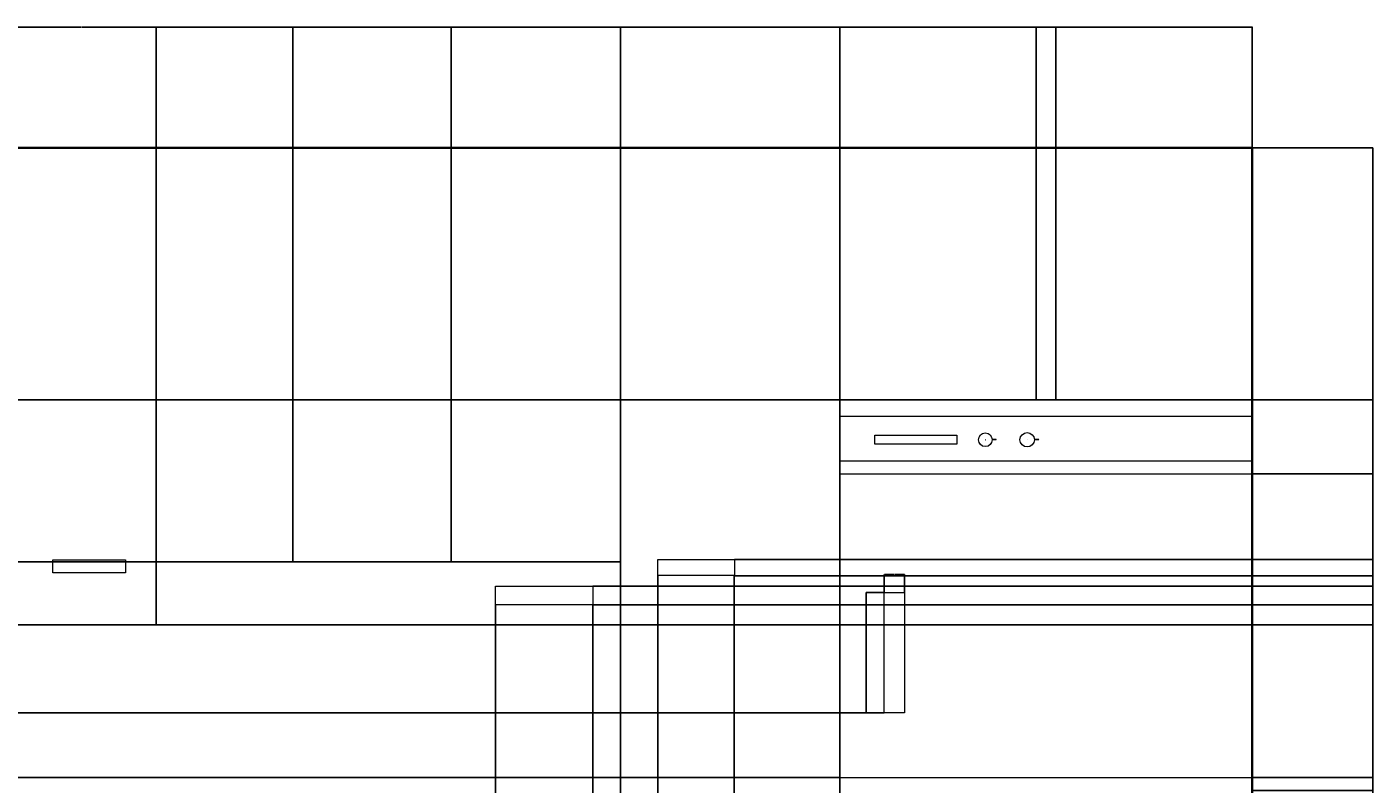
# Model space of a CAD drawing. Units: millimetres. Extents: x 4725 to 8727, y 2935 to 5260.
# Tile 3 of 3: x 6642 to 8727, y 4087 to 5260. Entities that reach past the tile are written whole.
import ezdxf

# ---------------------------------------------------------------- set-up
doc = ezdxf.new("R2010")
doc.units = ezdxf.units.MM
for name, color, linetype, lineweight in [('A-ANNO-DIMS', 2, 'Continuous', 18), ('A-CASE-HRDW', 9, 'Continuous', 13), ('A-ELEV', 7, 'Continuous', 35), ('A-EQPM', 4, 'Continuous', 18), ('A-FLOR-CASE', 8, 'Continuous', 25)]:
    doc.layers.add(name, color=color, linetype=linetype, lineweight=lineweight)
doc.styles.get("Standard").update_dxf_attribs({"font": 'arial.ttf'})
doc.dimstyles.get("Standard").update_dxf_attribs({"dimtxt": 0.18, "dimasz": 0.18, "dimexe": 0.18, "dimexo": 0.0625, "dimgap": 0.09, "dimtad": 0, "dimtih": 1, "dimtoh": 1, "dimdec": 4, "dimzin": 0, "dimdsep": 46, "dimtxsty": 'Standard', "dimcen": 0.09, "dimadec": 0, "dimazin": 0, "dimtfac": 1, "dimtdec": 4, "dimtofl": 0, "dimtmove": 0, "dimatfit": 3, "dimfxl": 1, "dimtolj": 1, "dimtzin": 0, "dimarcsym": 0})

# ---------------------------------------------------------------- blocks, each defined once
blk = doc.blocks.new('REFRIGERATOR-DOOR-PULL')
blk.add_lwpolyline([(0, 186.1), (31.3, 186.1), (31.3, 0), (0, 0)], close=True)
blk = doc.blocks.new('*D5')
at = {"layer": 'A-ANNO-DIMS', "color": 0, "lineweight": -2, "transparency": 16777216}
for p, q in [((7969.7, 4384.1), (7941.7, 4384.1)), ((7941.9, 4383.9), (7941.9, 4291.2)), ((7941.9, 4198.2), (7941.9, 4290.9)), ((7969.7, 4198), (7941.7, 4198))]:
    blk.add_line(p, q, dxfattribs=at)
at = {"layer": 'A-ANNO-DIMS', "color": 0, "transparency": 16777216}
for points in [[(7941.8, 4383.9), (7941.9, 4383.9), (7941.9, 4384.1)], [(7941.8, 4198.2), (7941.9, 4198.2), (7941.9, 4198)]]:
    blk.add_solid(points, dxfattribs=at)
at = {"layer": 'Defpoints', "color": 0, "transparency": 16777216}
for p in [(7941.9, 4384.1), (7969.8, 4384.1), (7969.8, 4198)]:
    blk.add_point(p, dxfattribs=at)
at = {"layer": 'A-ANNO-DIMS', "color": 0, "transparency": 16777216, "insert": (7941.9, 4291), "char_height": 0.18, "attachment_point": 5}
blk.add_mtext('\\A1;PULL 186 TYP.', dxfattribs=at)
blk = doc.blocks.new('*D6')
at = {"layer": 'A-ANNO-DIMS', "color": 0, "lineweight": -2, "transparency": 16777216}
for p, q in [((7969.8, 4384.1), (7969.8, 4412.2)), ((7969.9, 4412), (7984.9, 4412)), ((8000.9, 4412), (7985.9, 4412)), ((8001, 4384.1), (8001, 4412.2))]:
    blk.add_line(p, q, dxfattribs=at)
at = {"layer": 'A-ANNO-DIMS', "color": 0, "transparency": 16777216}
for points in [[(7969.9, 4412), (7969.9, 4412), (7969.8, 4412)], [(8000.9, 4412), (8000.9, 4412), (8001, 4412)]]:
    blk.add_solid(points, dxfattribs=at)
at = {"layer": 'Defpoints', "color": 0, "transparency": 16777216}
for p in [(8001, 4412), (7969.8, 4384.1), (8001, 4384.1)]:
    blk.add_point(p, dxfattribs=at)
at = {"layer": 'A-ANNO-DIMS', "color": 0, "transparency": 16777216, "insert": (7985.4, 4412), "char_height": 0.18, "attachment_point": 5}
blk.add_mtext('\\A1;31 TYP.', dxfattribs=at)
blk = doc.blocks.new('*D14')
at = {"layer": 'A-ANNO-DIMS', "color": 0, "lineweight": -2, "transparency": 16777216}
for p, q in [((6841.9, 5073.2), (6841.9, 5260.1)), ((6842.1, 5260), (6947.4, 5260)), ((7053.5, 5260), (6948.2, 5260)), ((7053.7, 5073.2), (7053.7, 5260.1))]:
    blk.add_line(p, q, dxfattribs=at)
at = {"layer": 'A-ANNO-DIMS', "color": 0, "transparency": 16777216}
for points in [[(6842.1, 5260), (6842.1, 5259.9), (6841.9, 5260)], [(7053.5, 5260), (7053.5, 5259.9), (7053.7, 5260)]]:
    blk.add_solid(points, dxfattribs=at)
at = {"layer": 'Defpoints', "color": 0, "transparency": 16777216}
for p in [(7053.7, 5260), (6841.9, 5073.1), (7053.7, 5073.1)]:
    blk.add_point(p, dxfattribs=at)
at = {"layer": 'A-ANNO-DIMS', "color": 0, "transparency": 16777216, "insert": (6947.8, 5260), "char_height": 0.18, "attachment_point": 5}
blk.add_mtext('\\A1;211.8', dxfattribs=at)
blk = doc.blocks.new('*D15')
at = {"layer": 'A-ANNO-DIMS', "color": 0, "lineweight": -2, "transparency": 16777216}
for p, q in [((7053.7, 5073.2), (7053.7, 5260.1)), ((7053.9, 5260), (7176, 5260)), ((7298.9, 5260), (7176.8, 5260)), ((7299.1, 5073.2), (7299.1, 5260.1))]:
    blk.add_line(p, q, dxfattribs=at)
at = {"layer": 'A-ANNO-DIMS', "color": 0, "transparency": 16777216}
for points in [[(7053.9, 5260), (7053.9, 5259.9), (7053.7, 5260)], [(7298.9, 5260), (7298.9, 5259.9), (7299.1, 5260)]]:
    blk.add_solid(points, dxfattribs=at)
at = {"layer": 'Defpoints', "color": 0, "transparency": 16777216}
for p in [(7299.1, 5260), (7053.7, 5073.1), (7299.1, 5073.1)]:
    blk.add_point(p, dxfattribs=at)
at = {"layer": 'A-ANNO-DIMS', "color": 0, "transparency": 16777216, "insert": (7176.4, 5260), "char_height": 0.18, "attachment_point": 5}
blk.add_mtext('\\A1;245.4', dxfattribs=at)
blk = doc.blocks.new('*D16')
at = {"layer": 'A-ANNO-DIMS', "color": 0, "lineweight": -2, "transparency": 16777216}
for p, q in [((7299.1, 5073.2), (7299.1, 5260.1)), ((7299.3, 5260), (7429.8, 5260)), ((7561.2, 5260), (7430.6, 5260)), ((7561.3, 5073.2), (7561.3, 5260.1))]:
    blk.add_line(p, q, dxfattribs=at)
at = {"layer": 'A-ANNO-DIMS', "color": 0, "transparency": 16777216}
for points in [[(7299.3, 5260), (7299.3, 5259.9), (7299.1, 5260)], [(7561.2, 5260), (7561.2, 5259.9), (7561.3, 5260)]]:
    blk.add_solid(points, dxfattribs=at)
at = {"layer": 'Defpoints', "color": 0, "transparency": 16777216}
for p in [(7561.3, 5260), (7299.1, 5073.1), (7561.3, 5073.1)]:
    blk.add_point(p, dxfattribs=at)
at = {"layer": 'A-ANNO-DIMS', "color": 0, "transparency": 16777216, "insert": (7430.2, 5260), "char_height": 0.18, "attachment_point": 5}
blk.add_mtext('\\A1;262.2', dxfattribs=at)
blk = doc.blocks.new('*D17')
at = {"layer": 'A-ANNO-DIMS', "color": 0, "lineweight": -2, "transparency": 16777216}
for p, q in [((7561.3, 5073.2), (7561.3, 5260.1)), ((7561.5, 5260), (7730.7, 5260)), ((7900.7, 5260), (7731.5, 5260)), ((7900.9, 5073.2), (7900.9, 5260.1))]:
    blk.add_line(p, q, dxfattribs=at)
at = {"layer": 'A-ANNO-DIMS', "color": 0, "transparency": 16777216}
for points in [[(7561.5, 5260), (7561.5, 5259.9), (7561.3, 5260)], [(7900.7, 5260), (7900.7, 5259.9), (7900.9, 5260)]]:
    blk.add_solid(points, dxfattribs=at)
at = {"layer": 'Defpoints', "color": 0, "transparency": 16777216}
for p in [(7900.9, 5260), (7561.3, 5073.1), (7900.9, 5073.1)]:
    blk.add_point(p, dxfattribs=at)
at = {"layer": 'A-ANNO-DIMS', "color": 0, "transparency": 16777216, "insert": (7731.1, 5260), "char_height": 0.18, "attachment_point": 5}
blk.add_mtext('\\A1;339.5', dxfattribs=at)
blk = doc.blocks.new('*D18')
at = {"layer": 'A-ANNO-DIMS', "color": 0, "lineweight": -2, "transparency": 16777216}
for p, q in [((7900.9, 5073.2), (7900.9, 5260.1)), ((7901, 5260), (8052.6, 5260)), ((8205, 5260), (8053.5, 5260)), ((8205.2, 5073.2), (8205.2, 5260.1))]:
    blk.add_line(p, q, dxfattribs=at)
at = {"layer": 'A-ANNO-DIMS', "color": 0, "transparency": 16777216}
for points in [[(7901, 5260), (7901, 5259.9), (7900.9, 5260)], [(8205, 5260), (8205, 5259.9), (8205.2, 5260)]]:
    blk.add_solid(points, dxfattribs=at)
at = {"layer": 'Defpoints', "color": 0, "transparency": 16777216}
for p in [(8205.2, 5260), (7900.9, 5073.1), (8205.2, 5073.1)]:
    blk.add_point(p, dxfattribs=at)
at = {"layer": 'A-ANNO-DIMS', "color": 0, "transparency": 16777216, "insert": (8053, 5260), "char_height": 0.18, "attachment_point": 5}
blk.add_mtext('\\A1;304.35', dxfattribs=at)
blk = doc.blocks.new('*D19')
at = {"layer": 'A-ANNO-DIMS', "color": 0, "lineweight": -2, "transparency": 16777216}
for p, q in [((8205.2, 5073.2), (8205.2, 5260.1)), ((8205.4, 5260), (8220, 5260)), ((8235, 5260), (8220.4, 5260)), ((8235.2, 5073.2), (8235.2, 5260.1))]:
    blk.add_line(p, q, dxfattribs=at)
at = {"layer": 'A-ANNO-DIMS', "color": 0, "transparency": 16777216}
for points in [[(8205.4, 5260), (8205.4, 5259.9), (8205.2, 5260)], [(8235, 5260), (8235, 5259.9), (8235.2, 5260)]]:
    blk.add_solid(points, dxfattribs=at)
at = {"layer": 'Defpoints', "color": 0, "transparency": 16777216}
for p in [(8235.2, 5260), (8205.2, 5073.1), (8235.2, 5073.1)]:
    blk.add_point(p, dxfattribs=at)
at = {"layer": 'A-ANNO-DIMS', "color": 0, "transparency": 16777216, "insert": (8220.2, 5260), "char_height": 0.18, "attachment_point": 5}
blk.add_mtext('\\A1;30', dxfattribs=at)
blk = doc.blocks.new('*D20')
at = {"layer": 'A-ANNO-DIMS', "color": 0, "lineweight": -2, "transparency": 16777216}
for p, q in [((8235.2, 5073.2), (8235.2, 5260.1)), ((8235.4, 5260), (8386.9, 5260)), ((8539.4, 5260), (8387.9, 5260)), ((8539.6, 5073.2), (8539.6, 5260.1))]:
    blk.add_line(p, q, dxfattribs=at)
at = {"layer": 'A-ANNO-DIMS', "color": 0, "transparency": 16777216}
for points in [[(8235.4, 5260), (8235.4, 5259.9), (8235.2, 5260)], [(8539.4, 5260), (8539.4, 5259.9), (8539.6, 5260)]]:
    blk.add_solid(points, dxfattribs=at)
at = {"layer": 'Defpoints', "color": 0, "transparency": 16777216}
for p in [(8539.6, 5260), (8235.2, 5073.1), (8539.6, 5073.1)]:
    blk.add_point(p, dxfattribs=at)
at = {"layer": 'A-ANNO-DIMS', "color": 0, "transparency": 16777216, "insert": (8387.4, 5260), "char_height": 0.18, "attachment_point": 5}
blk.add_mtext('\\A1;304.35', dxfattribs=at)
blk = doc.blocks.new('*D27')
at = {"layer": 'A-ANNO-DIMS', "color": 0, "lineweight": -2, "transparency": 16777216}
for p, q in [((8539.6, 4097.4), (8726.6, 4097.4)), ((8726.4, 4097.2), (8726.4, 4087.6)), ((8726.4, 4077.6), (8726.4, 4087.2)), ((8539.6, 4077.4), (8726.6, 4077.4))]:
    blk.add_line(p, q, dxfattribs=at)
at = {"layer": 'A-ANNO-DIMS', "color": 0, "transparency": 16777216}
for points in [[(8726.4, 4097.2), (8726.4, 4097.2), (8726.4, 4097.4)], [(8726.4, 4077.6), (8726.4, 4077.6), (8726.4, 4077.4)]]:
    blk.add_solid(points, dxfattribs=at)
at = {"layer": 'Defpoints', "color": 0, "transparency": 16777216}
for p in [(8539.6, 4097.4), (8726.4, 4097.4), (8539.6, 4077.4)]:
    blk.add_point(p, dxfattribs=at)
at = {"layer": 'A-ANNO-DIMS', "color": 0, "transparency": 16777216, "insert": (8726.4, 4087.4), "char_height": 0.18, "attachment_point": 5}
blk.add_mtext('\\A1;20', dxfattribs=at)
blk = doc.blocks.new('*D28')
at = {"layer": 'A-ANNO-DIMS', "color": 0, "lineweight": -2, "transparency": 16777216}
for p, q in [((8539.6, 4568), (8726.6, 4568)), ((8726.4, 4567.8), (8726.4, 4332.9)), ((8726.4, 4097.6), (8726.4, 4332.5)), ((8539.6, 4097.4), (8726.6, 4097.4))]:
    blk.add_line(p, q, dxfattribs=at)
at = {"layer": 'A-ANNO-DIMS', "color": 0, "transparency": 16777216}
for points in [[(8726.4, 4567.8), (8726.4, 4567.8), (8726.4, 4568)], [(8726.4, 4097.6), (8726.4, 4097.6), (8726.4, 4097.4)]]:
    blk.add_solid(points, dxfattribs=at)
at = {"layer": 'Defpoints', "color": 0, "transparency": 16777216}
for p in [(8539.6, 4568), (8539.6, 4097.4), (8726.4, 4097.4)]:
    blk.add_point(p, dxfattribs=at)
at = {"layer": 'A-ANNO-DIMS', "color": 0, "transparency": 16777216, "insert": (8726.4, 4332.7), "char_height": 0.18, "attachment_point": 5}
blk.add_mtext('\\A1;470.6', dxfattribs=at)
blk = doc.blocks.new('*D29')
at = {"layer": 'A-ANNO-DIMS', "color": 0, "lineweight": -2, "transparency": 16777216}
for p, q in [((8539.6, 4682.5), (8726.6, 4682.5)), ((8726.4, 4682.3), (8726.4, 4625.4)), ((8726.4, 4568.2), (8726.4, 4625)), ((8539.6, 4568), (8726.6, 4568))]:
    blk.add_line(p, q, dxfattribs=at)
at = {"layer": 'A-ANNO-DIMS', "color": 0, "transparency": 16777216}
for points in [[(8726.4, 4682.3), (8726.4, 4682.3), (8726.4, 4682.5)], [(8726.4, 4568.2), (8726.4, 4568.2), (8726.4, 4568)]]:
    blk.add_solid(points, dxfattribs=at)
at = {"layer": 'Defpoints', "color": 0, "transparency": 16777216}
for p in [(8539.6, 4682.5), (8726.4, 4682.5), (8539.6, 4568)]:
    blk.add_point(p, dxfattribs=at)
at = {"layer": 'A-ANNO-DIMS', "color": 0, "transparency": 16777216, "insert": (8726.4, 4625.2), "char_height": 0.18, "attachment_point": 5}
blk.add_mtext('\\A1;114.46', dxfattribs=at)
blk = doc.blocks.new('*D30')
at = {"layer": 'A-ANNO-DIMS', "color": 0, "lineweight": -2, "transparency": 16777216}
for p, q in [((8205.1, 5073.1), (4725.3, 5073.1)), ((4725.5, 5072.9), (4725.5, 4878)), ((4725.5, 4682.6), (4725.5, 4877.6)), ((7900.8, 4682.5), (4725.3, 4682.5))]:
    blk.add_line(p, q, dxfattribs=at)
at = {"layer": 'A-ANNO-DIMS', "color": 0, "transparency": 16777216}
for points in [[(4725.5, 5072.9), (4725.5, 5072.9), (4725.5, 5073.1)], [(4725.5, 4682.6), (4725.5, 4682.6), (4725.5, 4682.5)]]:
    blk.add_solid(points, dxfattribs=at)
at = {"layer": 'Defpoints', "color": 0, "transparency": 16777216}
for p in [(4725.5, 5073.1), (8205.2, 5073.1), (7900.9, 4682.5)]:
    blk.add_point(p, dxfattribs=at)
at = {"layer": 'A-ANNO-DIMS', "color": 0, "transparency": 16777216, "insert": (4725.5, 4877.8), "char_height": 0.18, "attachment_point": 5}
blk.add_mtext('\\A1;390.7', dxfattribs=at)
blk = doc.blocks.new('*D31')
at = {"layer": 'A-ANNO-DIMS', "color": 0, "lineweight": -2, "transparency": 16777216}
for p, q in [((6841.9, 4431.6), (4725.3, 4431.6)), ((4725.5, 4431.4), (4725.5, 4383.1)), ((4725.5, 4334.4), (4725.5, 4382.7)), ((6841.9, 4334.2), (4725.3, 4334.2))]:
    blk.add_line(p, q, dxfattribs=at)
at = {"layer": 'A-ANNO-DIMS', "color": 0, "transparency": 16777216}
for points in [[(4725.5, 4431.4), (4725.5, 4431.4), (4725.5, 4431.6)], [(4725.5, 4334.4), (4725.5, 4334.4), (4725.5, 4334.2)]]:
    blk.add_solid(points, dxfattribs=at)
at = {"layer": 'Defpoints', "color": 0, "transparency": 16777216}
for p in [(4725.5, 4431.6), (6841.9, 4431.6), (6841.9, 4334.2)]:
    blk.add_point(p, dxfattribs=at)
at = {"layer": 'A-ANNO-DIMS', "color": 0, "transparency": 16777216, "insert": (4725.5, 4382.9), "char_height": 0.18, "attachment_point": 5}
blk.add_mtext('\\A1;97.4', dxfattribs=at)
blk = doc.blocks.new('*D32')
at = {"layer": 'A-ANNO-DIMS', "color": 0, "lineweight": -2, "transparency": 16777216}
for p, q in [((7367.7, 4364.8), (7367.7, 2934.7)), ((7518.4, 4364.8), (7518.4, 2934.7)), ((7367.8, 2934.8), (7442.6, 2934.8)), ((7518.2, 2934.8), (7443.5, 2934.8))]:
    blk.add_line(p, q, dxfattribs=at)
at = {"layer": 'A-ANNO-DIMS', "color": 0, "transparency": 16777216}
for points in [[(7367.8, 2934.9), (7367.8, 2934.8), (7367.7, 2934.8)], [(7518.2, 2934.9), (7518.2, 2934.8), (7518.4, 2934.8)]]:
    blk.add_solid(points, dxfattribs=at)
at = {"layer": 'Defpoints', "color": 0, "transparency": 16777216}
for p in [(7367.7, 4364.8), (7518.4, 4364.8), (7518.4, 2934.8)]:
    blk.add_point(p, dxfattribs=at)
at = {"layer": 'A-ANNO-DIMS', "color": 0, "transparency": 16777216, "insert": (7443, 2934.8), "char_height": 0.18, "attachment_point": 5}
blk.add_mtext('\\A1;150.77', dxfattribs=at)
blk = doc.blocks.new('*D33')
at = {"layer": 'A-ANNO-DIMS', "color": 0, "lineweight": -2, "transparency": 16777216}
for p, q in [((7518.4, 4364.8), (7518.4, 2934.7)), ((7561.3, 4334.1), (7561.3, 2934.7)), ((7518.6, 2934.8), (7539.4, 2934.8)), ((7561.2, 2934.8), (7540.3, 2934.8))]:
    blk.add_line(p, q, dxfattribs=at)
at = {"layer": 'A-ANNO-DIMS', "color": 0, "transparency": 16777216}
for points in [[(7518.6, 2934.9), (7518.6, 2934.8), (7518.4, 2934.8)], [(7561.2, 2934.9), (7561.2, 2934.8), (7561.3, 2934.8)]]:
    blk.add_solid(points, dxfattribs=at)
at = {"layer": 'Defpoints', "color": 0, "transparency": 16777216}
for p in [(7518.4, 4364.8), (7561.3, 4334.2), (7561.3, 2934.8)]:
    blk.add_point(p, dxfattribs=at)
at = {"layer": 'A-ANNO-DIMS', "color": 0, "transparency": 16777216, "insert": (7539.9, 2934.8), "char_height": 0.18, "attachment_point": 5}
blk.add_mtext('\\A1;42.905', dxfattribs=at)
blk = doc.blocks.new('*D34')
at = {"layer": 'A-ANNO-DIMS', "color": 0, "lineweight": -2, "transparency": 16777216}
for p, q in [((7619, 4410.2), (7619, 2934.7)), ((7737.5, 4410.2), (7737.5, 2934.7)), ((7619.2, 2934.8), (7677.8, 2934.8)), ((7737.4, 2934.8), (7678.7, 2934.8))]:
    blk.add_line(p, q, dxfattribs=at)
at = {"layer": 'A-ANNO-DIMS', "color": 0, "transparency": 16777216}
for points in [[(7619.2, 2934.9), (7619.2, 2934.8), (7619, 2934.8)], [(7737.4, 2934.9), (7737.4, 2934.8), (7737.5, 2934.8)]]:
    blk.add_solid(points, dxfattribs=at)
at = {"layer": 'Defpoints', "color": 0, "transparency": 16777216}
for p in [(7619, 4410.2), (7737.5, 4410.2), (7737.5, 2934.8)]:
    blk.add_point(p, dxfattribs=at)
at = {"layer": 'A-ANNO-DIMS', "color": 0, "transparency": 16777216, "insert": (7678.3, 2934.8), "char_height": 0.18, "attachment_point": 5}
blk.add_mtext('\\A1;118.53', dxfattribs=at)
blk = doc.blocks.new('*D35')
at = {"layer": 'A-ANNO-DIMS', "color": 0, "lineweight": -2, "transparency": 16777216}
for p, q in [((7737.5, 4410.2), (7737.5, 2934.7)), ((7900.9, 4334.1), (7900.9, 2934.7)), ((7737.7, 2934.8), (7818.7, 2934.8)), ((7900.7, 2934.8), (7819.7, 2934.8))]:
    blk.add_line(p, q, dxfattribs=at)
at = {"layer": 'A-ANNO-DIMS', "color": 0, "transparency": 16777216}
for points in [[(7737.7, 2934.9), (7737.7, 2934.8), (7737.5, 2934.8)], [(7900.7, 2934.9), (7900.7, 2934.8), (7900.9, 2934.8)]]:
    blk.add_solid(points, dxfattribs=at)
at = {"layer": 'Defpoints', "color": 0, "transparency": 16777216}
for p in [(7737.5, 4410.2), (7900.9, 4334.2), (7900.9, 2934.8)]:
    blk.add_point(p, dxfattribs=at)
at = {"layer": 'A-ANNO-DIMS', "color": 0, "transparency": 16777216, "insert": (7819.2, 2934.8), "char_height": 0.18, "attachment_point": 5}
blk.add_mtext('\\A1;163.32', dxfattribs=at)
blk = doc.blocks.new('*D36')
at = {"layer": 'A-ANNO-DIMS', "color": 0, "lineweight": -2, "transparency": 16777216}
for p, q in [((7737.6, 4435.1), (8726.6, 4435.1)), ((8726.4, 4434.9), (8726.4, 4422.8)), ((8726.4, 4410.4), (8726.4, 4422.5)), ((7737.6, 4410.2), (8726.6, 4410.2))]:
    blk.add_line(p, q, dxfattribs=at)
at = {"layer": 'A-ANNO-DIMS', "color": 0, "transparency": 16777216}
for points in [[(8726.4, 4434.9), (8726.4, 4434.9), (8726.4, 4435.1)], [(8726.4, 4410.4), (8726.4, 4410.4), (8726.4, 4410.2)]]:
    blk.add_solid(points, dxfattribs=at)
at = {"layer": 'Defpoints', "color": 0, "transparency": 16777216}
for p in [(7737.5, 4435.1), (8726.4, 4435.1), (7737.5, 4410.2)]:
    blk.add_point(p, dxfattribs=at)
at = {"layer": 'A-ANNO-DIMS', "color": 0, "transparency": 16777216, "insert": (8726.4, 4422.7), "char_height": 0.18, "attachment_point": 5}
blk.add_mtext('\\A1;24.846', dxfattribs=at)
blk = doc.blocks.new('*D37')
at = {"layer": 'A-ANNO-DIMS', "color": 0, "lineweight": -2, "transparency": 16777216}
for p, q in [((7737.6, 4410.2), (8726.6, 4410.2)), ((8726.4, 4410.1), (8726.4, 4372.4)), ((8726.4, 4334.4), (8726.4, 4372)), ((7900.9, 4334.2), (8726.6, 4334.2))]:
    blk.add_line(p, q, dxfattribs=at)
at = {"layer": 'A-ANNO-DIMS', "color": 0, "transparency": 16777216}
for points in [[(8726.4, 4410.1), (8726.4, 4410.1), (8726.4, 4410.2)], [(8726.4, 4334.4), (8726.4, 4334.4), (8726.4, 4334.2)]]:
    blk.add_solid(points, dxfattribs=at)
at = {"layer": 'Defpoints', "color": 0, "transparency": 16777216}
for p in [(7737.5, 4410.2), (8726.4, 4410.2), (7900.9, 4334.2)]:
    blk.add_point(p, dxfattribs=at)
at = {"layer": 'A-ANNO-DIMS', "color": 0, "transparency": 16777216, "insert": (8726.4, 4372.2), "char_height": 0.18, "attachment_point": 5}
blk.add_mtext('\\A1;76.04', dxfattribs=at)
blk = doc.blocks.new('*D38')
at = {"layer": 'A-ANNO-DIMS', "color": 0, "lineweight": -2, "transparency": 16777216}
for p, q in [((7518.5, 4394.2), (8726.6, 4394.2)), ((8726.4, 4394), (8726.4, 4379.7)), ((8726.4, 4365), (8726.4, 4379.3)), ((7518.5, 4364.8), (8726.6, 4364.8))]:
    blk.add_line(p, q, dxfattribs=at)
at = {"layer": 'A-ANNO-DIMS', "color": 0, "transparency": 16777216}
for points in [[(8726.4, 4394), (8726.4, 4394), (8726.4, 4394.2)], [(8726.4, 4365), (8726.4, 4365), (8726.4, 4364.8)]]:
    blk.add_solid(points, dxfattribs=at)
at = {"layer": 'Defpoints', "color": 0, "transparency": 16777216}
for p in [(7518.4, 4394.2), (8726.4, 4394.2), (7518.4, 4364.8)]:
    blk.add_point(p, dxfattribs=at)
at = {"layer": 'A-ANNO-DIMS', "color": 0, "transparency": 16777216, "insert": (8726.4, 4379.5), "char_height": 0.18, "attachment_point": 5}
blk.add_mtext('\\A1;29.33', dxfattribs=at)
blk = doc.blocks.new('*D39')
at = {"layer": 'A-ANNO-DIMS', "color": 0, "lineweight": -2, "transparency": 16777216}
for p, q in [((7518.5, 4364.8), (8726.6, 4364.8)), ((8726.4, 4364.6), (8726.4, 4349.7)), ((8726.4, 4334.4), (8726.4, 4349.3)), ((7561.4, 4334.2), (8726.6, 4334.2))]:
    blk.add_line(p, q, dxfattribs=at)
at = {"layer": 'A-ANNO-DIMS', "color": 0, "transparency": 16777216}
for points in [[(8726.4, 4364.6), (8726.4, 4364.6), (8726.4, 4364.8)], [(8726.4, 4334.4), (8726.4, 4334.4), (8726.4, 4334.2)]]:
    blk.add_solid(points, dxfattribs=at)
at = {"layer": 'Defpoints', "color": 0, "transparency": 16777216}
for p in [(7518.4, 4364.8), (8726.4, 4364.8), (7561.3, 4334.2)]:
    blk.add_point(p, dxfattribs=at)
at = {"layer": 'A-ANNO-DIMS', "color": 0, "transparency": 16777216, "insert": (8726.4, 4349.5), "char_height": 0.18, "attachment_point": 5}
blk.add_mtext('\\A1;30.63', dxfattribs=at)
blk = doc.blocks.new('*D40')
at = {"layer": 'A-ANNO-DIMS', "color": 0, "lineweight": -2, "transparency": 16777216}
for p, q in [((4912.4, 5073.2), (4912.4, 5260.1)), ((4912.5, 5260), (6725.6, 5260)), ((8539.4, 5260), (6726.3, 5260)), ((8539.6, 5073.2), (8539.6, 5260.1))]:
    blk.add_line(p, q, dxfattribs=at)
at = {"layer": 'A-ANNO-DIMS', "color": 0, "transparency": 16777216}
for points in [[(4912.5, 5260), (4912.5, 5259.9), (4912.4, 5260)], [(8539.4, 5260), (8539.4, 5259.9), (8539.6, 5260)]]:
    blk.add_solid(points, dxfattribs=at)
at = {"layer": 'Defpoints', "color": 0, "transparency": 16777216}
for p in [(8539.6, 5260), (4912.4, 5073.1), (8539.6, 5073.1)]:
    blk.add_point(p, dxfattribs=at)
at = {"layer": 'A-ANNO-DIMS', "color": 0, "transparency": 16777216, "insert": (6726, 5260), "char_height": 0.18, "attachment_point": 5}
blk.add_mtext('\\A1;3627', dxfattribs=at)
blk = doc.blocks.new('*D41')
at = {"layer": 'A-ANNO-DIMS', "color": 0, "lineweight": -2, "transparency": 16777216}
for p, q in [((4912.4, 5073.1), (8726.6, 5073.1)), ((8726.4, 5072.9), (8726.4, 4097.6)), ((8726.4, 3121.9), (8726.4, 4097.2)), ((8539.6, 3121.7), (8726.6, 3121.7))]:
    blk.add_line(p, q, dxfattribs=at)
at = {"layer": 'A-ANNO-DIMS', "color": 0, "transparency": 16777216}
for points in [[(8726.4, 5072.9), (8726.4, 5072.9), (8726.4, 5073.1)], [(8726.4, 3121.9), (8726.4, 3121.9), (8726.4, 3121.7)]]:
    blk.add_solid(points, dxfattribs=at)
at = {"layer": 'Defpoints', "color": 0, "transparency": 16777216}
for p in [(4912.4, 5073.1), (8726.4, 5073.1), (8539.6, 3121.7)]:
    blk.add_point(p, dxfattribs=at)
at = {"layer": 'A-ANNO-DIMS', "color": 0, "transparency": 16777216, "insert": (8726.4, 4097.4), "char_height": 0.18, "attachment_point": 5}
blk.add_mtext('\\A1;1951.4', dxfattribs=at)
blk = doc.blocks.new('*D43')
at = {"layer": 'A-ANNO-DIMS', "color": 0, "lineweight": -2, "transparency": 16777216}
for p, q in [((7969.7, 4198), (4725.3, 4198)), ((4725.5, 4197.8), (4725.5, 4147.9)), ((4725.5, 4097.6), (4725.5, 4147.5)), ((7900.8, 4097.4), (4725.3, 4097.4))]:
    blk.add_line(p, q, dxfattribs=at)
at = {"layer": 'A-ANNO-DIMS', "color": 0, "transparency": 16777216}
for points in [[(4725.5, 4197.8), (4725.5, 4197.8), (4725.5, 4198)], [(4725.5, 4097.6), (4725.5, 4097.6), (4725.5, 4097.4)]]:
    blk.add_solid(points, dxfattribs=at)
at = {"layer": 'Defpoints', "color": 0, "transparency": 16777216}
for p in [(4725.5, 4198), (7969.8, 4198), (7900.9, 4097.4)]:
    blk.add_point(p, dxfattribs=at)
at = {"layer": 'A-ANNO-DIMS', "color": 0, "transparency": 16777216, "insert": (4725.5, 4147.7), "char_height": 0.18, "attachment_point": 5}
blk.add_mtext('\\A1;100.6', dxfattribs=at)
blk = doc.blocks.new('*D45')
at = {"layer": 'A-ANNO-DIMS', "color": 0, "lineweight": -2, "transparency": 16777216}
for p, q in [((8126.2, 4620.7), (8126.3, 4620.7)), ((8126.3, 4620.6), (8126.3, 4620.8)), ((8143.2, 4621.2), (8137, 4621))]:
    blk.add_line(p, q, dxfattribs=at)
at = {"layer": 'A-ANNO-DIMS', "color": 0, "transparency": 16777216}
blk.add_solid([(8137, 4621), (8137, 4621), (8136.9, 4621)], dxfattribs=at)
at = {"layer": 'Defpoints', "color": 0, "transparency": 16777216}
for p in [(8115.6, 4620.4), (8136.9, 4621)]:
    blk.add_point(p, dxfattribs=at)
at = {"layer": 'A-ANNO-DIMS', "color": 0, "transparency": 16777216, "insert": (8143.7, 4621.2), "char_height": 0.18, "attachment_point": 5}
blk.add_mtext('\\A1;∅21.23', dxfattribs=at)
blk = doc.blocks.new('*D46')
at = {"layer": 'A-ANNO-DIMS', "color": 0, "lineweight": -2, "transparency": 16777216}
for p, q in [((8191, 4620.7), (8191.2, 4620.7)), ((8191.1, 4620.6), (8191.1, 4620.8)), ((8208.9, 4621.2), (8202.4, 4621))]:
    blk.add_line(p, q, dxfattribs=at)
at = {"layer": 'A-ANNO-DIMS', "color": 0, "transparency": 16777216}
blk.add_solid([(8202.4, 4621), (8202.4, 4621), (8202.2, 4621)], dxfattribs=at)
at = {"layer": 'Defpoints', "color": 0, "transparency": 16777216}
for p in [(8179.9, 4620.4), (8202.2, 4621)]:
    blk.add_point(p, dxfattribs=at)
at = {"layer": 'A-ANNO-DIMS', "color": 0, "transparency": 16777216, "insert": (8209.5, 4621.2), "char_height": 0.18, "attachment_point": 5}
blk.add_mtext('\\A1;∅22.293', dxfattribs=at)

msp = doc.modelspace()

# ---------------------------------------------------------------- linework, layer by layer
at = {"layer": 'A-CASE-HRDW'}
for points in [[(6681.8901, 4434.9434), (6794.3549, 4434.9434), (6794.3549, 4414.8177), (6681.8901, 4414.8177)], [(7619.0046, 4435.0803), (7737.5372, 4435.0803), (7737.5372, 4410.2347), (7619.0046, 4410.2347)], [(7367.6547, 4394.1518), (7518.4266, 4394.1518), (7518.4266, 4364.8232), (7367.6547, 4364.8232)]]:
    msp.add_lwpolyline(points, close=True, dxfattribs=at)
at = {"layer": 'A-ELEV'}
for p, q in [((4912.3658, 5073.1177), (8539.5662, 5073.1177)), ((8539.5662, 5073.1177), (8539.5662, 3121.6884))]:
    msp.add_line(p, q, dxfattribs=at)
at = {"layer": 'A-EQPM'}
for p, q in [((7900.8562, 4657.4503), (8539.5662, 4657.4503)), ((7900.8562, 4587.9855), (8539.5662, 4587.9855)), ((7900.8562, 4567.9855), (8539.5662, 4567.9855)), ((7900.8562, 4097.4031), (8539.5662, 4097.4031))]:
    msp.add_line(p, q, dxfattribs=at)
msp.add_lwpolyline([(7955.1974, 4627.598), (8082.1625, 4627.598), (8082.1625, 4613.7977), (7955.1974, 4613.7977)], close=True, dxfattribs=at)
for centre, radius in [((8126.255, 4620.6979), 10.6156), ((8191.0657, 4620.6979), 11.1463)]:
    msp.add_circle(centre, radius, dxfattribs=at)
at = {"layer": 'A-FLOR-CASE'}
for p, q in [((6031.7891, 5073.1177), (6841.9423, 5073.1177)), ((6841.9423, 5073.1177), (6841.9423, 4334.1944)), ((7053.7251, 4431.5979), (7053.7251, 5073.1177)), ((7053.7251, 5073.1177), (7299.1242, 5073.1177)), ((7299.1242, 5073.1177), (7299.1242, 4431.5979)), ((7561.3315, 4431.5979), (7561.3315, 5073.1177)), ((7900.8562, 5073.1177), (7900.8562, 3121.6884)), ((8205.2112, 4682.4503), (8205.2112, 5073.1177)), ((8235.2112, 4682.4503), (8235.2112, 5073.1177)), ((7900.8562, 4682.4503), (8539.5662, 4682.4503)), ((6841.9423, 4431.5979), (7561.3315, 4431.5979)), ((7561.3315, 4431.5979), (7561.3315, 4334.1944)), ((6841.9423, 4334.1944), (6031.7891, 4334.1944)), ((6841.9423, 4334.1944), (7561.3315, 4334.1944)), ((7561.3315, 4334.1944), (7900.8562, 4334.1944))]:
    msp.add_line(p, q, dxfattribs=at)

# ---------------------------------------------------------------- block references
at = {"layer": 'A-EQPM'}
msp.add_blockref('REFRIGERATOR-DOOR-PULL', (7969.768, 4197.999), dxfattribs=at)

# ---------------------------------------------------------------- dimensions: what is measured, and where the dimension line sits
at = {"layer": 'A-ANNO-DIMS'}
for base, p1, p2, override, picture, middle in [((8539.5662, 5259.9677), (4912.3658, 5073.1177), (8539.5662, 5073.1177), {"dimdec": 0, "dimlfac": 1, "dimrnd": 0, "dimzin": 0, "dimdsep": 46, "dimlunit": 2}, '*D40', (6725.966, 5259.9677)), ((7053.7251, 5259.9677), (6841.9423, 5073.1177), (7053.7251, 5073.1177), {"dimdec": 1, "dimlfac": 1, "dimrnd": 0, "dimzin": 0, "dimdsep": 46, "dimlunit": 2}, '*D14', (6947.8337, 5259.9677)), ((7299.1242, 5259.9677), (7053.7251, 5073.1177), (7299.1242, 5073.1177), {"dimdec": 1, "dimlfac": 1, "dimrnd": 0, "dimzin": 0, "dimdsep": 46, "dimlunit": 2}, '*D15', (7176.4246, 5259.9677)), ((7561.3315, 5259.9677), (7299.1242, 5073.1177), (7561.3315, 5073.1177), {"dimdec": 1, "dimlfac": 1, "dimrnd": 0, "dimzin": 0, "dimdsep": 46, "dimlunit": 2}, '*D16', (7430.2278, 5259.9677)), ((7900.8562, 5259.9677), (7561.3315, 5073.1177), (7900.8562, 5073.1177), {"dimdec": 1, "dimlfac": 1, "dimrnd": 0, "dimzin": 0, "dimdsep": 46, "dimlunit": 2}, '*D17', (7731.0938, 5259.9677)), ((8205.211232, 5259.967732), (7900.856234, 5073.117732), (8205.211232, 5073.117732), {"dimdec": 2, "dimlfac": 1, "dimrnd": 0, "dimzin": 0, "dimdsep": 46, "dimlunit": 2}, '*D18', (8053.033733, 5259.967732)), ((8235.2112, 5259.9677), (8205.2112, 5073.1177), (8235.2112, 5073.1177), {"dimdec": 0, "dimlfac": 1, "dimrnd": 0, "dimzin": 0, "dimdsep": 46, "dimlunit": 2}, '*D19', (8220.2112, 5259.9677)), ((8539.566231, 5259.967732), (8235.211232, 5073.117732), (8539.566231, 5073.117732), {"dimdec": 2, "dimlfac": 1, "dimrnd": 0, "dimzin": 0, "dimdsep": 46, "dimlunit": 2}, '*D20', (8387.388731, 5259.967732)), ((7737.5372, 2934.8384), (7619.0046, 4410.2347), (7737.5372, 4410.2347), {"dimdec": 2, "dimlfac": 1, "dimrnd": 0, "dimzin": 0, "dimdsep": 46, "dimlunit": 2}, '*D34', (7678.2709, 2934.8384)), ((7900.8562, 2934.8384), (7737.5372, 4410.2347), (7900.8562, 4334.1944), {"dimdec": 2, "dimlfac": 1, "dimrnd": 0, "dimzin": 0, "dimdsep": 46, "dimlunit": 2}, '*D35', (7819.1967, 2934.8384)), ((7518.4266, 2934.8384), (7367.6547, 4364.8232), (7518.4266, 4364.8232), {"dimdec": 2, "dimlfac": 1, "dimrnd": 0, "dimzin": 0, "dimdsep": 46, "dimlunit": 2}, '*D32', (7443.0406, 2934.8384)), ((7561.3315, 2934.8384), (7518.4266, 4364.8232), (7561.3315, 4334.1944), {"dimdec": 3, "dimlfac": 1, "dimrnd": 0, "dimzin": 0, "dimdsep": 46, "dimlunit": 2}, '*D33', (7539.879, 2934.8384))]:
    dim = msp.add_linear_dim(base=base, p1=p1, p2=p2, dimstyle='Standard', override=override, dxfattribs=at)
    dim.commit()
    dim.dimension.update_dxf_attribs({"geometry": picture, "text_midpoint": middle})
for base, p1, p2, override, picture, middle in [((4725.5158, 5073.1177), (7900.8562, 4682.4503), (8205.2112, 5073.1177), {"dimdec": 1, "dimlfac": 1, "dimrnd": 0, "dimzin": 0, "dimdsep": 46, "dimlunit": 2}, '*D30', (4725.5158, 4877.784)), ((8726.4162, 5073.1177), (8539.5662, 3121.6884), (4912.3658, 5073.1177), {"dimdec": 1, "dimlfac": 1, "dimrnd": 0, "dimzin": 0, "dimdsep": 46, "dimlunit": 2}, '*D41', (8726.4162, 4097.4031)), ((8726.4162, 4682.4503), (8539.5662, 4567.9855), (8539.5662, 4682.4503), {"dimdec": 2, "dimlfac": 1, "dimrnd": 0, "dimzin": 0, "dimdsep": 46, "dimlunit": 2}, '*D29', (8726.4162, 4625.2179)), ((8726.4162, 4097.4031), (8539.5662, 4567.9855), (8539.5662, 4097.4031), {"dimdec": 1, "dimlfac": 1, "dimrnd": 0, "dimzin": 0, "dimdsep": 46, "dimlunit": 2}, '*D28', (8726.4162, 4332.6943)), ((4725.5158, 4431.5979), (6841.9423, 4334.1944), (6841.9423, 4431.5979), {"dimdec": 1, "dimlfac": 1, "dimrnd": 0, "dimzin": 0, "dimdsep": 46, "dimlunit": 2}, '*D31', (4725.5158, 4382.8962)), ((8726.4162, 4435.0803), (7737.5372, 4410.2347), (7737.5372, 4435.0803), {"dimdec": 3, "dimlfac": 1, "dimrnd": 0, "dimzin": 0, "dimdsep": 46, "dimlunit": 2}, '*D36', (8726.4162, 4422.6575)), ((8726.4162, 4410.2347), (7900.8562, 4334.1944), (7737.5372, 4410.2347), {"dimdec": 2, "dimlfac": 1, "dimrnd": 0, "dimzin": 0, "dimdsep": 46, "dimlunit": 2}, '*D37', (8726.4162, 4372.2146)), ((8726.4162, 4394.1518), (7518.4266, 4364.8232), (7518.4266, 4394.1518), {"dimdec": 2, "dimlfac": 1, "dimrnd": 0, "dimzin": 0, "dimdsep": 46, "dimlunit": 2}, '*D38', (8726.4162, 4379.4875)), ((8726.4162, 4364.8232), (7561.3315, 4334.1944), (7518.4266, 4364.8232), {"dimdec": 2, "dimlfac": 1, "dimrnd": 0, "dimzin": 0, "dimdsep": 46, "dimlunit": 2}, '*D39', (8726.4162, 4349.5088)), ((4725.5158, 4197.9992), (7900.8562, 4097.4031), (7969.7678, 4197.9992), {"dimdec": 1, "dimlfac": 1, "dimrnd": 0, "dimzin": 0, "dimdsep": 46, "dimlunit": 2}, '*D43', (4725.5158, 4147.7011)), ((8726.4162, 4097.4031), (8539.5662, 4077.4031), (8539.5662, 4097.4031), {"dimdec": 0, "dimlfac": 1, "dimrnd": 0, "dimzin": 0, "dimdsep": 46, "dimlunit": 2}, '*D27', (8726.4162, 4087.4031))]:
    dim = msp.add_linear_dim(base=base, p1=p1, p2=p2, angle=90, dimstyle='Standard', override=override, dxfattribs=at)
    dim.commit()
    dim.dimension.update_dxf_attribs({"geometry": picture, "text_midpoint": middle})
for p1, p2, override, picture, middle in [((8115.6438, 4620.3938), (8136.8662, 4621.0019), {"dimdec": 2, "dimlfac": 1, "dimrnd": 0, "dimzin": 0, "dimdsep": 46, "dimlunit": 2}, '*D45', (8143.233, 4621.1843)), ((8179.9235, 4620.3928), (8202.2079, 4621.003), {"dimdec": 3, "dimlfac": 1, "dimrnd": 0, "dimzin": 0, "dimdsep": 46, "dimlunit": 2}, '*D46', (8208.8932, 4621.186))]:
    dim = msp.add_diameter_dim_2p(p1=p1, p2=p2, dimstyle='Standard', override=override, dxfattribs=at)
    dim.commit()
    dim.dimension.update_dxf_attribs({"geometry": picture, "text_midpoint": middle, "dimtype": 163})
dim = msp.add_linear_dim(base=(8001.0347, 4411.9934), p1=(7969.7678, 4384.0811), p2=(8001.0347, 4384.0811), text='<> TYP.', dimstyle='Standard', override={"dimdec": 0, "dimlfac": 1, "dimrnd": 0, "dimzin": 0, "dimdsep": 46, "dimlunit": 2}, dxfattribs=at)
dim.commit()
dim.dimension.update_dxf_attribs({"geometry": '*D6', "text_midpoint": (7985.4013, 4411.9934)})
dim = msp.add_linear_dim(base=(7941.8555, 4384.0811), p1=(7969.7678, 4197.9992), p2=(7969.7678, 4384.0811), angle=90, text='PULL <> TYP.', dimstyle='Standard', override={"dimdec": 0, "dimlfac": 1, "dimrnd": 0, "dimzin": 0, "dimdsep": 46, "dimlunit": 2}, dxfattribs=at)
dim.commit()
dim.dimension.update_dxf_attribs({"geometry": '*D5', "text_midpoint": (7941.8555, 4291.0401)})

doc.saveas('drawing.dxf')
